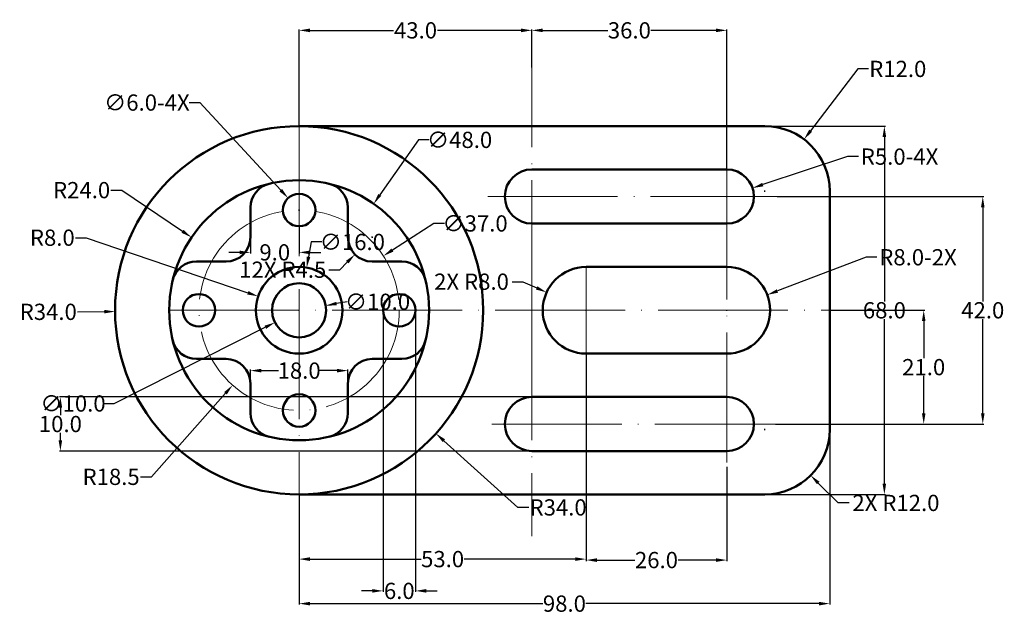
# Model space of a CAD drawing. Units: inches. Extents: x 173 to 355, y 91 to 201.
import ezdxf

# ---------------------------------------------------------------- set-up
doc = ezdxf.new("R2010")
doc.units = ezdxf.units.IN
doc.header["$MEASUREMENT"] = 0
doc.linetypes.add('ACAD_ISO04W100', pattern=[30, 24, -3, 0, -3])
for name, color, linetype, lineweight in [('M-CNTR', 4, 'ACAD_ISO04W100', 18), ('M-DIMS', 2, 'Continuous', 25), ('M-OUTL', 7, 'Continuous', 50)]:
    doc.layers.add(name, color=color, linetype=linetype, lineweight=lineweight)
doc.styles.get("Standard").update_dxf_attribs({"font": 'arial.ttf'})
doc.dimstyles.get("Standard").update_dxf_attribs({"dimtxt": 3, "dimasz": 2, "dimexe": 0.18, "dimexo": 0.0625, "dimgap": 0.09, "dimtad": 0, "dimtih": 1, "dimtoh": 1, "dimdec": 1, "dimzin": 0, "dimdsep": 46, "dimtxsty": 'Standard', "dimcen": 0.09, "dimclrd": 1, "dimclre": 1, "dimadec": 0, "dimazin": 0, "dimtfac": 1, "dimtdec": 1, "dimtofl": 0, "dimtmove": 0, "dimatfit": 3, "dimfxl": 1, "dimtolj": 1, "dimtzin": 0, "dimarcsym": 0})

# ---------------------------------------------------------------- blocks, each defined once
blk = doc.blocks.new('*U1')
blk.add_circle((0, 0), 3)
blk = doc.blocks.new('*U2')
at = {"layer": 'M-OUTL', "color": 0, "linetype": 'ByBlock', "lineweight": -2, "transparency": 16777216}
blk.add_blockref('*U1', (224.3, 165.64), dxfattribs=at)
for p, rotation in [((205.8, 147.14), 90), ((242.8, 147.14), 270), ((224.3, 128.64), 180)]:
    blk.add_blockref('*U1', p, dxfattribs=dict(at, rotation=rotation))
blk = doc.blocks.new('*D3')
at = {"layer": 'Defpoints', "color": 0, "transparency": 16777216}
for p in [(303.3, 198.82), (267.3, 191.92), (303.3, 173.14)]:
    blk.add_point(p, dxfattribs=at)
at = {"layer": 'M-DIMS', "color": 0, "lineweight": -2, "transparency": 16777216}
for p, q in [((267.3, 191.99), (267.3, 199)), ((269.3, 198.82), (281.32, 198.82)), ((301.3, 198.82), (289.28, 198.82)), ((303.3, 173.21), (303.3, 199))]:
    blk.add_line(p, q, dxfattribs=at)
at = {"layer": 'M-DIMS', "color": 0, "transparency": 16777216}
for points in [[(269.3, 199.15), (269.3, 198.48), (267.3, 198.82)], [(301.3, 199.15), (301.3, 198.48), (303.3, 198.82)]]:
    blk.add_solid(points, dxfattribs=at)
at = {"layer": 'M-DIMS', "color": 0, "transparency": 16777216, "insert": (285.3, 198.82), "char_height": 3, "attachment_point": 5}
blk.add_mtext('\\A1;36.0', dxfattribs=at)
blk = doc.blocks.new('*D4')
at = {"layer": 'Defpoints', "color": 0, "transparency": 16777216}
for p in [(267.3, 198.82), (267.3, 191.92), (224.3, 181.14)]:
    blk.add_point(p, dxfattribs=at)
at = {"layer": 'M-DIMS', "color": 0, "lineweight": -2, "transparency": 16777216}
for p, q in [((224.3, 181.21), (224.3, 199)), ((226.3, 198.82), (241.76, 198.82)), ((265.3, 198.82), (249.84, 198.82)), ((267.3, 191.99), (267.3, 199))]:
    blk.add_line(p, q, dxfattribs=at)
at = {"layer": 'M-DIMS', "color": 0, "transparency": 16777216}
for points in [[(226.3, 199.15), (226.3, 198.48), (224.3, 198.82)], [(265.3, 199.15), (265.3, 198.48), (267.3, 198.82)]]:
    blk.add_solid(points, dxfattribs=at)
at = {"layer": 'M-DIMS', "color": 0, "transparency": 16777216, "insert": (245.8, 198.82), "char_height": 3, "attachment_point": 5}
blk.add_mtext('\\A1;43.0', dxfattribs=at)
blk = doc.blocks.new('*D5')
at = {"layer": 'Defpoints', "color": 0, "transparency": 16777216}
for p in [(277.3, 139.14), (224.3, 113.14), (277.3, 101.2)]:
    blk.add_point(p, dxfattribs=at)
at = {"layer": 'M-DIMS', "color": 0, "lineweight": -2, "transparency": 16777216}
for p, q in [((277.3, 139.08), (277.3, 101.02)), ((224.3, 113.08), (224.3, 101.02)), ((226.3, 101.2), (246.82, 101.2)), ((275.3, 101.2), (254.78, 101.2))]:
    blk.add_line(p, q, dxfattribs=at)
at = {"layer": 'M-DIMS', "color": 0, "transparency": 16777216}
for points in [[(226.3, 101.53), (226.3, 100.86), (224.3, 101.2)], [(275.3, 101.53), (275.3, 100.86), (277.3, 101.2)]]:
    blk.add_solid(points, dxfattribs=at)
at = {"layer": 'M-DIMS', "color": 0, "transparency": 16777216, "insert": (250.8, 101.2), "char_height": 3, "attachment_point": 5}
blk.add_mtext('\\A1;53.0', dxfattribs=at)
blk = doc.blocks.new('*D6')
at = {"layer": 'Defpoints', "color": 0, "transparency": 16777216}
for p in [(277.3, 139.14), (303.3, 118.29), (303.3, 101.02)]:
    blk.add_point(p, dxfattribs=at)
at = {"layer": 'M-DIMS', "color": 0, "lineweight": -2, "transparency": 16777216}
for p, q in [((277.3, 139.08), (277.3, 100.84)), ((303.3, 118.22), (303.3, 100.84)), ((279.3, 101.02), (286.29, 101.02)), ((301.3, 101.02), (294.31, 101.02))]:
    blk.add_line(p, q, dxfattribs=at)
at = {"layer": 'M-DIMS', "color": 0, "transparency": 16777216}
for points in [[(279.3, 101.35), (279.3, 100.68), (277.3, 101.02)], [(301.3, 101.35), (301.3, 100.68), (303.3, 101.02)]]:
    blk.add_solid(points, dxfattribs=at)
at = {"layer": 'M-DIMS', "color": 0, "transparency": 16777216, "insert": (290.3, 101.02), "char_height": 3, "attachment_point": 5}
blk.add_mtext('\\A1;26.0', dxfattribs=at)
blk = doc.blocks.new('*D7')
at = {"layer": 'Defpoints', "color": 0, "transparency": 16777216}
for p in [(322.3, 125.14), (224.3, 113.14), (322.3, 92.98)]:
    blk.add_point(p, dxfattribs=at)
at = {"layer": 'M-DIMS', "color": 0, "lineweight": -2, "transparency": 16777216}
for p, q in [((322.3, 125.08), (322.3, 92.8)), ((224.3, 113.08), (224.3, 92.8)), ((226.3, 92.98), (269.32, 92.98)), ((320.3, 92.98), (277.28, 92.98))]:
    blk.add_line(p, q, dxfattribs=at)
at = {"layer": 'M-DIMS', "color": 0, "transparency": 16777216}
for points in [[(226.3, 93.31), (226.3, 92.64), (224.3, 92.98)], [(320.3, 93.31), (320.3, 92.64), (322.3, 92.98)]]:
    blk.add_solid(points, dxfattribs=at)
at = {"layer": 'M-DIMS', "color": 0, "transparency": 16777216, "insert": (273.3, 92.98), "char_height": 3, "attachment_point": 5}
blk.add_mtext('\\A1;98.0', dxfattribs=at)
blk = doc.blocks.new('*D8')
at = {"layer": 'Defpoints', "color": 0, "transparency": 16777216}
for p in [(310.78, 149.99), (303.3, 147.14)]:
    blk.add_point(p, dxfattribs=at)
at = {"layer": 'M-DIMS', "color": 0, "lineweight": -2, "transparency": 16777216}
for p, q in [((329.02, 156.93), (312.65, 150.7)), ((331.02, 156.93), (329.02, 156.93)), ((303.21, 147.14), (303.39, 147.14)), ((303.3, 147.05), (303.3, 147.23))]:
    blk.add_line(p, q, dxfattribs=at)
at = {"layer": 'M-DIMS', "color": 0, "transparency": 16777216}
blk.add_solid([(312.53, 151.01), (312.76, 150.39), (310.78, 149.99)], dxfattribs=at)
at = {"layer": 'M-DIMS', "color": 0, "transparency": 16777216, "insert": (338.62, 156.93), "char_height": 3, "attachment_point": 5}
blk.add_mtext('\\A1;R8.0-2X', dxfattribs=at)
blk = doc.blocks.new('*D9')
at = {"layer": 'Defpoints', "color": 0, "transparency": 16777216}
for p in [(317.57, 178.69), (310.3, 169.14)]:
    blk.add_point(p, dxfattribs=at)
at = {"layer": 'M-DIMS', "color": 0, "lineweight": -2, "transparency": 16777216}
for p, q in [((327.47, 191.7), (318.78, 180.28)), ((329.47, 191.7), (327.47, 191.7)), ((310.3, 169.05), (310.3, 169.23)), ((310.21, 169.14), (310.39, 169.14))]:
    blk.add_line(p, q, dxfattribs=at)
at = {"layer": 'M-DIMS', "color": 0, "transparency": 16777216}
blk.add_solid([(318.51, 180.49), (319.04, 180.08), (317.57, 178.69)], dxfattribs=at)
at = {"layer": 'M-DIMS', "color": 0, "transparency": 16777216, "insert": (334.88, 191.7), "char_height": 3, "attachment_point": 5}
blk.add_mtext('\\A1;R12.0', dxfattribs=at)
blk = doc.blocks.new('*D10')
at = {"layer": 'Defpoints', "color": 0, "transparency": 16777216}
for p in [(308.05, 169.71), (303.3, 168.14)]:
    blk.add_point(p, dxfattribs=at)
at = {"layer": 'M-DIMS', "color": 0, "lineweight": -2, "transparency": 16777216}
for p, q in [((325.61, 175.51), (309.95, 170.34)), ((327.61, 175.51), (325.61, 175.51)), ((303.21, 168.14), (303.39, 168.14)), ((303.3, 168.05), (303.3, 168.23))]:
    blk.add_line(p, q, dxfattribs=at)
at = {"layer": 'M-DIMS', "color": 0, "transparency": 16777216}
blk.add_solid([(309.84, 170.66), (310.05, 170.02), (308.05, 169.71)], dxfattribs=at)
at = {"layer": 'M-DIMS', "color": 0, "transparency": 16777216, "insert": (335.21, 175.51), "char_height": 3, "attachment_point": 5}
blk.add_mtext('\\A1;R5.0-4X', dxfattribs=at)
blk = doc.blocks.new('*D11')
at = {"layer": 'Defpoints', "color": 0, "transparency": 16777216}
for p in [(312.52, 168.14), (312.26, 126.14), (350.58, 126.14)]:
    blk.add_point(p, dxfattribs=at)
at = {"layer": 'M-DIMS', "color": 0, "lineweight": -2, "transparency": 16777216}
for p, q in [((312.58, 168.14), (350.76, 168.14)), ((350.58, 166.14), (350.58, 148.77)), ((350.58, 128.14), (350.58, 145.52)), ((312.32, 126.14), (350.76, 126.14))]:
    blk.add_line(p, q, dxfattribs=at)
at = {"layer": 'M-DIMS', "color": 0, "transparency": 16777216}
for points in [[(350.25, 166.14), (350.91, 166.14), (350.58, 168.14)], [(350.25, 128.14), (350.91, 128.14), (350.58, 126.14)]]:
    blk.add_solid(points, dxfattribs=at)
at = {"layer": 'M-DIMS', "color": 0, "transparency": 16777216, "insert": (350.58, 147.14), "char_height": 3, "attachment_point": 5}
blk.add_mtext('\\A1;42.0', dxfattribs=at)
blk = doc.blocks.new('*D12')
at = {"layer": 'Defpoints', "color": 0, "transparency": 16777216}
for p in [(322.3, 147.14), (312.26, 126.14), (339.67, 126.14)]:
    blk.add_point(p, dxfattribs=at)
at = {"layer": 'M-DIMS', "color": 0, "lineweight": -2, "transparency": 16777216}
for p, q in [((322.36, 147.14), (339.85, 147.14)), ((339.67, 145.14), (339.67, 138.27)), ((339.67, 128.14), (339.67, 135.02)), ((312.32, 126.14), (339.85, 126.14))]:
    blk.add_line(p, q, dxfattribs=at)
at = {"layer": 'M-DIMS', "color": 0, "transparency": 16777216}
for points in [[(339.34, 145.14), (340, 145.14), (339.67, 147.14)], [(339.34, 128.14), (340, 128.14), (339.67, 126.14)]]:
    blk.add_solid(points, dxfattribs=at)
at = {"layer": 'M-DIMS', "color": 0, "transparency": 16777216, "insert": (339.67, 136.64), "char_height": 3, "attachment_point": 5}
blk.add_mtext('\\A1;21.0', dxfattribs=at)
blk = doc.blocks.new('*D13')
at = {"layer": 'Defpoints', "color": 0, "transparency": 16777216}
for p in [(224.3, 162.64), (215.3, 160.64), (224.3, 157.83)]:
    blk.add_point(p, dxfattribs=at)
at = {"layer": 'M-DIMS', "color": 0, "lineweight": -2, "transparency": 16777216}
for p, q in [((224.3, 162.58), (224.3, 157.65)), ((215.3, 160.58), (215.3, 157.65)), ((213.3, 157.83), (211.3, 157.83)), ((226.3, 157.83), (228.3, 157.83))]:
    blk.add_line(p, q, dxfattribs=at)
at = {"layer": 'M-DIMS', "color": 0, "transparency": 16777216}
for points in [[(213.3, 158.16), (213.3, 157.49), (215.3, 157.83)], [(226.3, 158.16), (226.3, 157.49), (224.3, 157.83)]]:
    blk.add_solid(points, dxfattribs=at)
at = {"layer": 'M-DIMS', "color": 0, "transparency": 16777216, "insert": (219.8, 157.83), "char_height": 3, "attachment_point": 5}
blk.add_mtext('\\A1;9.0', dxfattribs=at)
blk = doc.blocks.new('*D14')
at = {"layer": 'Defpoints', "color": 0, "transparency": 16777216}
for p in [(222.26, 167.85), (226.33, 163.44)]:
    blk.add_point(p, dxfattribs=at)
at = {"layer": 'M-DIMS', "color": 0, "lineweight": -2, "transparency": 16777216}
for p, q in [((203.97, 185.49), (205.97, 185.49)), ((205.97, 185.49), (220.91, 169.32)), ((224.21, 165.64), (224.39, 165.64)), ((224.3, 165.55), (224.3, 165.73))]:
    blk.add_line(p, q, dxfattribs=at)
at = {"layer": 'M-DIMS', "color": 0, "transparency": 16777216}
blk.add_solid([(221.15, 169.54), (220.66, 169.09), (222.26, 167.85)], dxfattribs=at)
at = {"layer": 'M-DIMS', "color": 0, "transparency": 16777216, "insert": (196.18, 185.49), "char_height": 3, "attachment_point": 5}
blk.add_mtext('\\A1;∅6.0-4X', dxfattribs=at)
blk = doc.blocks.new('*D15')
at = {"layer": 'Defpoints', "color": 0, "transparency": 16777216}
for p in [(204.42, 160.6), (224.3, 147.14)]:
    blk.add_point(p, dxfattribs=at)
at = {"layer": 'M-DIMS', "color": 0, "lineweight": -2, "transparency": 16777216}
for p, q in [((189.54, 169.32), (191.54, 169.32)), ((191.54, 169.32), (202.77, 161.72)), ((224.21, 147.14), (224.39, 147.14)), ((224.3, 147.05), (224.3, 147.23))]:
    blk.add_line(p, q, dxfattribs=at)
at = {"layer": 'M-DIMS', "color": 0, "transparency": 16777216}
blk.add_solid([(202.95, 161.99), (202.58, 161.44), (204.42, 160.6)], dxfattribs=at)
at = {"layer": 'M-DIMS', "color": 0, "transparency": 16777216, "insert": (184.12, 169.32), "char_height": 3, "attachment_point": 5}
blk.add_mtext('\\A1;R24.0', dxfattribs=at)
blk = doc.blocks.new('*D16')
at = {"layer": 'Defpoints', "color": 0, "transparency": 16777216}
for p in [(190.3, 146.9), (224.3, 147.14)]:
    blk.add_point(p, dxfattribs=at)
at = {"layer": 'M-DIMS', "color": 0, "lineweight": -2, "transparency": 16777216}
for p, q in [((183.37, 146.85), (188.3, 146.89)), ((224.21, 147.14), (224.39, 147.14)), ((224.3, 147.05), (224.3, 147.23))]:
    blk.add_line(p, q, dxfattribs=at)
at = {"layer": 'M-DIMS', "color": 0, "transparency": 16777216}
blk.add_solid([(188.3, 147.22), (188.3, 146.56), (190.3, 146.9)], dxfattribs=at)
at = {"layer": 'M-DIMS', "color": 0, "transparency": 16777216, "insert": (177.96, 146.85), "char_height": 3, "attachment_point": 5}
blk.add_mtext('\\A1;R34.0', dxfattribs=at)
blk = doc.blocks.new('*D17')
at = {"layer": 'Defpoints', "color": 0, "transparency": 16777216}
for p in [(224.3, 147.14), (212.02, 133.31)]:
    blk.add_point(p, dxfattribs=at)
at = {"layer": 'M-DIMS', "color": 0, "lineweight": -2, "transparency": 16777216}
for p, q in [((224.21, 147.14), (224.39, 147.14)), ((224.3, 147.05), (224.3, 147.23)), ((197, 116.39), (210.69, 131.81)), ((195, 116.39), (197, 116.39))]:
    blk.add_line(p, q, dxfattribs=at)
at = {"layer": 'M-DIMS', "color": 0, "transparency": 16777216}
blk.add_solid([(210.44, 132.03), (210.94, 131.59), (212.02, 133.31)], dxfattribs=at)
at = {"layer": 'M-DIMS', "color": 0, "transparency": 16777216, "insert": (189.57, 116.39), "char_height": 3, "attachment_point": 5}
blk.add_mtext('\\A1;R18.5', dxfattribs=at)
blk = doc.blocks.new('*D18')
at = {"layer": 'Defpoints', "color": 0, "transparency": 16777216}
for p in [(216.73, 149.72), (224.3, 147.14)]:
    blk.add_point(p, dxfattribs=at)
at = {"layer": 'M-DIMS', "color": 0, "lineweight": -2, "transparency": 16777216}
for p, q in [((182.96, 160.54), (184.96, 160.54)), ((184.96, 160.54), (214.83, 150.37)), ((224.21, 147.14), (224.39, 147.14)), ((224.3, 147.05), (224.3, 147.23))]:
    blk.add_line(p, q, dxfattribs=at)
at = {"layer": 'M-DIMS', "color": 0, "transparency": 16777216}
blk.add_solid([(214.94, 150.68), (214.72, 150.05), (216.73, 149.72)], dxfattribs=at)
at = {"layer": 'M-DIMS', "color": 0, "transparency": 16777216, "insert": (178.71, 160.54), "char_height": 3, "attachment_point": 5}
blk.add_mtext('\\A1;R8.0', dxfattribs=at)
blk = doc.blocks.new('*D19')
at = {"layer": 'Defpoints', "color": 0, "transparency": 16777216}
for p in [(228.76, 149.39), (219.83, 144.89)]:
    blk.add_point(p, dxfattribs=at)
at = {"layer": 'M-DIMS', "color": 0, "lineweight": -2, "transparency": 16777216}
for p, q in [((224.21, 147.14), (224.39, 147.14)), ((224.3, 147.05), (224.3, 147.23)), ((190.14, 129.93), (218.05, 143.99)), ((188.14, 129.93), (190.14, 129.93))]:
    blk.add_line(p, q, dxfattribs=at)
at = {"layer": 'M-DIMS', "color": 0, "transparency": 16777216}
blk.add_solid([(217.9, 144.29), (218.2, 143.7), (219.83, 144.89)], dxfattribs=at)
at = {"layer": 'M-DIMS', "color": 0, "transparency": 16777216, "insert": (182.53, 129.93), "char_height": 3, "attachment_point": 5}
blk.add_mtext('\\A1;∅10.0', dxfattribs=at)
blk = doc.blocks.new('*D20')
at = {"layer": 'Defpoints', "color": 0, "transparency": 16777216}
for p in [(233.3, 136), (215.3, 133.64), (233.3, 133.64)]:
    blk.add_point(p, dxfattribs=at)
at = {"layer": 'M-DIMS', "color": 0, "lineweight": -2, "transparency": 16777216}
for p, q in [((215.3, 133.71), (215.3, 136.18)), ((217.3, 136), (220.46, 136)), ((231.3, 136), (228.14, 136)), ((233.3, 133.71), (233.3, 136.18))]:
    blk.add_line(p, q, dxfattribs=at)
at = {"layer": 'M-DIMS', "color": 0, "transparency": 16777216}
for points in [[(217.3, 136.33), (217.3, 135.66), (215.3, 136)], [(231.3, 136.33), (231.3, 135.66), (233.3, 136)]]:
    blk.add_solid(points, dxfattribs=at)
at = {"layer": 'M-DIMS', "color": 0, "transparency": 16777216, "insert": (224.3, 136), "char_height": 3, "attachment_point": 5}
blk.add_mtext('\\A1;18.0', dxfattribs=at)
blk = doc.blocks.new('HUB-INTERLOBE-RELIEF')
for p, q in [((3.46, 7.96), (3.46, 13.44)), ((7.96, 3.46), (13.44, 3.46))]:
    blk.add_line(p, q)
for centre, start, end in [((-1.04, 13.44), 0, 76.6576), ((7.96, 7.96), 180, 270), ((13.44, -1.04), 13.3424, 90)]:
    blk.add_arc(centre, 4.5, start, end)
blk = doc.blocks.new('GUIDE-SLOT-NARROW')
blk.add_lwpolyline([(41, 10), (5, 10, 1), (5, 0), (41, 0, 1)], format="xyb", close=True)
blk = doc.blocks.new('*D23')
at = {"layer": 'Defpoints', "color": 0, "transparency": 16777216}
for p in [(310.3, 181.14), (310.3, 113.14), (332.4, 113.14)]:
    blk.add_point(p, dxfattribs=at)
at = {"layer": 'M-DIMS', "color": 1, "lineweight": -2, "transparency": 16777216}
for p, q in [((310.36, 181.14), (332.58, 181.14)), ((332.4, 179.14), (332.4, 148.77)), ((332.4, 115.14), (332.4, 145.52)), ((310.36, 113.14), (332.58, 113.14))]:
    blk.add_line(p, q, dxfattribs=at)
at = {"layer": 'M-DIMS', "color": 1, "transparency": 16777216}
for points in [[(332.07, 179.14), (332.73, 179.14), (332.4, 181.14)], [(332.07, 115.14), (332.73, 115.14), (332.4, 113.14)]]:
    blk.add_solid(points, dxfattribs=at)
at = {"layer": 'M-DIMS', "color": 0, "transparency": 16777216, "insert": (332.4, 147.14), "char_height": 3, "attachment_point": 5}
blk.add_mtext('\\A1;68.0', dxfattribs=at)
blk = doc.blocks.new('*D24')
at = {"layer": 'Defpoints', "color": 0, "transparency": 16777216}
for p in [(239.8, 147.14), (245.8, 147.14), (245.8, 95.33)]:
    blk.add_point(p, dxfattribs=at)
at = {"layer": 'M-DIMS', "color": 1, "lineweight": -2, "transparency": 16777216}
for p, q in [((239.8, 147.08), (239.8, 95.15)), ((245.8, 147.08), (245.8, 95.15)), ((237.8, 95.33), (235.8, 95.33)), ((247.8, 95.33), (249.8, 95.33))]:
    blk.add_line(p, q, dxfattribs=at)
at = {"layer": 'M-DIMS', "color": 1, "transparency": 16777216}
for points in [[(237.8, 95.67), (237.8, 95), (239.8, 95.33)], [(247.8, 95.67), (247.8, 95), (245.8, 95.33)]]:
    blk.add_solid(points, dxfattribs=at)
at = {"layer": 'M-DIMS', "color": 0, "transparency": 16777216, "insert": (242.8, 95.33), "char_height": 3, "attachment_point": 5}
blk.add_mtext('\\A1;6.0', dxfattribs=at)
blk = doc.blocks.new('*D25')
at = {"layer": 'Defpoints', "color": 0, "transparency": 16777216}
for p in [(180.2, 131.14), (267.3, 131.14), (267.3, 121.14)]:
    blk.add_point(p, dxfattribs=at)
at = {"layer": 'M-DIMS', "color": 1, "lineweight": -2, "transparency": 16777216}
for p, q in [((267.24, 131.14), (180.02, 131.14)), ((180.2, 129.14), (180.2, 127.77)), ((180.2, 123.14), (180.2, 124.52)), ((267.24, 121.14), (180.02, 121.14))]:
    blk.add_line(p, q, dxfattribs=at)
at = {"layer": 'M-DIMS', "color": 1, "transparency": 16777216}
for points in [[(179.87, 129.14), (180.53, 129.14), (180.2, 131.14)], [(179.87, 123.14), (180.53, 123.14), (180.2, 121.14)]]:
    blk.add_solid(points, dxfattribs=at)
at = {"layer": 'M-DIMS', "color": 0, "transparency": 16777216, "insert": (180.2, 126.14), "char_height": 3, "attachment_point": 5}
blk.add_mtext('\\A1;10.0', dxfattribs=at)
blk = doc.blocks.new('*D26')
at = {"layer": 'Defpoints', "color": 0, "transparency": 16777216}
for p in [(224.3, 147.14), (249.56, 124.39)]:
    blk.add_point(p, dxfattribs=at)
at = {"layer": 'M-DIMS', "color": 1, "lineweight": -2, "transparency": 16777216}
for p, q in [((224.21, 147.14), (224.39, 147.14)), ((224.3, 147.05), (224.3, 147.23)), ((264.72, 110.74), (251.05, 123.05)), ((266.72, 110.74), (264.72, 110.74))]:
    blk.add_line(p, q, dxfattribs=at)
at = {"layer": 'M-DIMS', "color": 1, "transparency": 16777216}
blk.add_solid([(251.27, 123.3), (250.83, 122.8), (249.56, 124.39)], dxfattribs=at)
at = {"layer": 'M-DIMS', "color": 0, "transparency": 16777216, "insert": (272.14, 110.74), "char_height": 3, "attachment_point": 5}
blk.add_mtext('\\A1;R34.0', dxfattribs=at)
blk = doc.blocks.new('*D27')
at = {"layer": 'Defpoints', "color": 0, "transparency": 16777216}
for p in [(238.06, 166.8), (210.53, 127.48)]:
    blk.add_point(p, dxfattribs=at)
at = {"layer": 'M-DIMS', "color": 1, "lineweight": -2, "transparency": 16777216}
for p, q in [((246.32, 178.6), (239.21, 168.44)), ((248.32, 178.6), (246.32, 178.6)), ((224.21, 147.14), (224.39, 147.14)), ((224.3, 147.05), (224.3, 147.23))]:
    blk.add_line(p, q, dxfattribs=at)
at = {"layer": 'M-DIMS', "color": 1, "transparency": 16777216}
blk.add_solid([(238.94, 168.63), (239.48, 168.25), (238.06, 166.8)], dxfattribs=at)
at = {"layer": 'M-DIMS', "color": 0, "transparency": 16777216, "insert": (253.94, 178.6), "char_height": 3, "attachment_point": 5}
blk.add_mtext('\\A1;∅48.0', dxfattribs=at)
blk = doc.blocks.new('*D28')
at = {"layer": 'Defpoints', "color": 0, "transparency": 16777216}
for p in [(239.85, 157.16), (208.75, 137.13)]:
    blk.add_point(p, dxfattribs=at)
at = {"layer": 'M-DIMS', "color": 1, "lineweight": -2, "transparency": 16777216}
for p, q in [((249.18, 163.17), (241.53, 158.25)), ((251.18, 163.17), (249.18, 163.17)), ((224.21, 147.14), (224.39, 147.14)), ((224.3, 147.05), (224.3, 147.23))]:
    blk.add_line(p, q, dxfattribs=at)
at = {"layer": 'M-DIMS', "color": 1, "transparency": 16777216}
blk.add_solid([(241.35, 158.53), (241.71, 157.97), (239.85, 157.16)], dxfattribs=at)
at = {"layer": 'M-DIMS', "color": 0, "transparency": 16777216, "insert": (256.8, 163.17), "char_height": 3, "attachment_point": 5}
blk.add_mtext('\\A1;∅37.0', dxfattribs=at)
blk = doc.blocks.new('*D29')
at = {"layer": 'Defpoints', "color": 0, "transparency": 16777216}
for p in [(225.69, 155.02), (222.91, 139.27)]:
    blk.add_point(p, dxfattribs=at)
at = {"layer": 'M-DIMS', "color": 1, "lineweight": -2, "transparency": 16777216}
for p, q in [((226.52, 159.75), (226.04, 156.99)), ((228.52, 159.75), (226.52, 159.75)), ((224.21, 147.14), (224.39, 147.14)), ((224.3, 147.05), (224.3, 147.23))]:
    blk.add_line(p, q, dxfattribs=at)
at = {"layer": 'M-DIMS', "color": 1, "transparency": 16777216}
blk.add_solid([(225.71, 157.05), (226.36, 156.93), (225.69, 155.02)], dxfattribs=at)
at = {"layer": 'M-DIMS', "color": 0, "transparency": 16777216, "insert": (234.13, 159.75), "char_height": 3, "attachment_point": 5}
blk.add_mtext('\\A1;∅16.0', dxfattribs=at)
blk = doc.blocks.new('*D30')
at = {"layer": 'Defpoints', "color": 0, "transparency": 16777216}
for p in [(229.22, 148.01), (219.37, 146.28)]:
    blk.add_point(p, dxfattribs=at)
at = {"layer": 'M-DIMS', "color": 1, "lineweight": -2, "transparency": 16777216}
for p, q in [((233.16, 148.71), (231.19, 148.36)), ((224.21, 147.14), (224.39, 147.14)), ((224.3, 147.05), (224.3, 147.23))]:
    blk.add_line(p, q, dxfattribs=at)
at = {"layer": 'M-DIMS', "color": 1, "transparency": 16777216}
blk.add_solid([(231.13, 148.69), (231.25, 148.03), (229.22, 148.01)], dxfattribs=at)
at = {"layer": 'M-DIMS', "color": 0, "transparency": 16777216, "insert": (238.78, 148.71), "char_height": 3, "attachment_point": 5}
blk.add_mtext('\\A1;∅10.0', dxfattribs=at)
blk = doc.blocks.new('*D31')
at = {"layer": 'Defpoints', "color": 0, "transparency": 16777216}
for p in [(237.8, 160.64), (234.62, 157.46)]:
    blk.add_point(p, dxfattribs=at)
at = {"layer": 'M-DIMS', "color": 1, "lineweight": -2, "transparency": 16777216}
for p, q in [((237.71, 160.64), (237.89, 160.64)), ((237.8, 160.55), (237.8, 160.73)), ((229.79, 154.63), (231.79, 154.63)), ((231.79, 154.63), (233.2, 156.05))]:
    blk.add_line(p, q, dxfattribs=at)
at = {"layer": 'M-DIMS', "color": 1, "transparency": 16777216}
blk.add_solid([(232.97, 156.28), (233.44, 155.81), (234.62, 157.46)], dxfattribs=at)
at = {"layer": 'M-DIMS', "color": 0, "transparency": 16777216, "insert": (221.27, 154.63), "char_height": 3, "attachment_point": 5}
blk.add_mtext('\\A1;12X R4.5', dxfattribs=at)
blk = doc.blocks.new('*D32')
at = {"layer": 'Defpoints', "color": 0, "transparency": 16777216}
for p in [(310.3, 125.14), (318.78, 116.66)]:
    blk.add_point(p, dxfattribs=at)
at = {"layer": 'M-DIMS', "color": 1, "lineweight": -2, "transparency": 16777216}
for p, q in [((310.21, 125.14), (310.39, 125.14)), ((310.3, 125.05), (310.3, 125.23)), ((323.88, 111.57), (320.2, 115.24)), ((325.88, 111.57), (323.88, 111.57))]:
    blk.add_line(p, q, dxfattribs=at)
at = {"layer": 'M-DIMS', "color": 1, "transparency": 16777216}
blk.add_solid([(320.43, 115.48), (319.96, 115.01), (318.78, 116.66)], dxfattribs=at)
at = {"layer": 'M-DIMS', "color": 0, "transparency": 16777216, "insert": (334.54, 111.57), "char_height": 3, "attachment_point": 5}
blk.add_mtext('\\A1;2X R12.0', dxfattribs=at)
blk = doc.blocks.new('*D33')
at = {"layer": 'Defpoints', "color": 0, "transparency": 16777216}
for p in [(270.01, 150.44), (277.3, 147.14)]:
    blk.add_point(p, dxfattribs=at)
at = {"layer": 'M-DIMS', "color": 1, "lineweight": -2, "transparency": 16777216}
for p, q in [((263.64, 152.42), (265.64, 152.42)), ((265.64, 152.42), (268.19, 151.27)), ((277.21, 147.14), (277.39, 147.14)), ((277.3, 147.05), (277.3, 147.23))]:
    blk.add_line(p, q, dxfattribs=at)
at = {"layer": 'M-DIMS', "color": 1, "transparency": 16777216}
blk.add_solid([(268.33, 151.57), (268.05, 150.97), (270.01, 150.44)], dxfattribs=at)
at = {"layer": 'M-DIMS', "color": 0, "transparency": 16777216, "insert": (256.14, 152.42), "char_height": 3, "attachment_point": 5}
blk.add_mtext('\\A1;2X R8.0', dxfattribs=at)

msp = doc.modelspace()

# ---------------------------------------------------------------- linework, layer by layer
at = {"layer": 'M-CNTR'}
for p, q in [((267.3, 147.14), (267.3, 191.92)), ((224.3, 181.14), (224.3, 113.14)), ((303.3, 173.14), (303.3, 118.29)), ((259.13, 168.14), (312.52, 168.14)), ((277.3, 155.14), (277.3, 139.14)), ((200.3, 147.14), (322.3, 147.14)), ((267.3, 147.14), (267.3, 105.43)), ((259.88, 126.14), (312.26, 126.14))]:
    msp.add_line(p, q, dxfattribs=at)
msp.add_circle((224.3, 147.14), 18.5, dxfattribs=at)
at = {"layer": 'M-OUTL'}
for p, q in [((224.3, 181.14), (310.3, 181.14)), ((322.3, 125.14), (322.3, 169.14)), ((277.3, 155.14), (303.3, 155.14)), ((277.3, 139.14), (303.3, 139.14)), ((224.3, 113.14), (310.3, 113.14))]:
    msp.add_line(p, q, dxfattribs=at)
for radius in [34, 24, 8, 5]:
    msp.add_circle((224.3, 147.14), radius, dxfattribs=at)
for centre, radius, start, end in [((310.3, 169.14), 12, 0, 90), ((277.3, 147.14), 8, 90, 270), ((303.3, 147.14), 8, 270, 90), ((310.3, 125.14), 12, 270, 0)]:
    msp.add_arc(centre, radius, start, end, dxfattribs=at)

# ---------------------------------------------------------------- block references
for name, p in [('GUIDE-SLOT-NARROW', (262.3, 163.14)), ('HUB-INTERLOBE-RELIEF', (229.84, 152.68)), ('*U2', (0, 0))]:
    msp.add_blockref(name, p, dxfattribs=at)
for p, rotation in [((218.76, 152.68), 89.99999999999974), ((218.76, 141.61), 180), ((229.84, 141.61), 269.9999999999998)]:
    msp.add_blockref('HUB-INTERLOBE-RELIEF', p, dxfattribs=dict(at, rotation=rotation))
at = {"layer": 'M-OUTL', "extrusion": (0, 0, -1), "zscale": -1, "rotation": 180}
msp.add_blockref('GUIDE-SLOT-NARROW', (-262.3, 131.14), dxfattribs=at)

# ---------------------------------------------------------------- dimensions: what is measured, and where the dimension line sits
at = {"layer": 'M-DIMS'}
for base, p1, p2, override, picture, middle in [((267.3, 198.82), (224.3, 181.14), (267.3, 191.92), {"dimclrd": 0, "dimclre": 0, "dimclrt": 0}, '*D4', (245.8, 198.82)), ((303.3, 198.82), (267.3, 191.92), (303.3, 173.14), {"dimclrd": 0, "dimclre": 0, "dimclrt": 0}, '*D3', (285.3, 198.82)), ((224.3, 157.83), (215.3, 160.64), (224.3, 162.64), {"dimclrd": 0, "dimclre": 0, "dimclrt": 0}, '*D13', (219.8, 157.83)), ((245.8, 95.33), (239.8, 147.14), (245.8, 147.14), {"dimdec": 1, "dimlfac": 1, "dimrnd": 0, "dimzin": 0, "dimdsep": 46, "dimlunit": 2}, '*D24', (242.8, 95.33)), ((277.3, 101.2), (224.3, 113.14), (277.3, 139.14), {"dimclrd": 0, "dimclre": 0, "dimclrt": 0}, '*D5', (250.8, 101.2)), ((303.3, 101.02), (277.3, 139.14), (303.3, 118.29), {"dimclrd": 0, "dimclre": 0, "dimclrt": 0}, '*D6', (290.3, 101.02)), ((233.3, 136), (215.3, 133.64), (233.3, 133.64), {"dimclrd": 0, "dimclre": 0, "dimclrt": 0}, '*D20', (224.3, 136)), ((322.3, 92.98), (224.3, 113.14), (322.3, 125.14), {"dimclrd": 0, "dimclre": 0, "dimclrt": 0}, '*D7', (273.3, 92.98))]:
    dim = msp.add_linear_dim(base=base, p1=p1, p2=p2, dimstyle='Standard', override=override, dxfattribs=at)
    dim.commit()
    dim.dimension.update_dxf_attribs({"geometry": picture, "text_midpoint": middle})
for center, mpoint, override, picture, middle in [((310.3, 169.14), (317.57, 178.69), {"dimclrd": 0, "dimclre": 0, "dimclrt": 0}, '*D9', (334.88, 191.7)), ((224.3, 147.14), (204.42, 160.6), {"dimclrd": 0, "dimclre": 0, "dimclrt": 0}, '*D15', (184.12, 169.32)), ((224.3, 147.14), (216.73, 149.72), {"dimclrd": 0, "dimclre": 0, "dimclrt": 0}, '*D18', (178.71, 160.54)), ((224.3, 147.14), (190.3, 146.9), {"dimclrd": 0, "dimclre": 0, "dimclrt": 0}, '*D16', (183.37, 146.85)), ((224.3, 147.14), (212.02, 133.31), {"dimclrd": 0, "dimclre": 0, "dimclrt": 0}, '*D17', (189.57, 116.39)), ((224.3, 147.14), (249.56, 124.39), {"dimdec": 1, "dimlfac": 1, "dimrnd": 0, "dimzin": 0, "dimdsep": 46, "dimlunit": 2}, '*D26', (272.14, 110.74))]:
    dim = msp.add_radius_dim(center=center, mpoint=mpoint, dimstyle='Standard', override=override, dxfattribs=at)
    dim.commit()
    dim.dimension.update_dxf_attribs({"geometry": picture, "text_midpoint": middle, "dimtype": 164})
dim = msp.add_diameter_dim_2p(p1=(226.33, 163.44), p2=(222.26, 167.85), text='<>-4X', dimstyle='Standard', override={"dimclrd": 0, "dimclre": 0, "dimclrt": 0}, dxfattribs=at)
dim.commit()
dim.dimension.update_dxf_attribs({"geometry": '*D14', "text_midpoint": (196.18, 185.49), "dimtype": 163})
for p1, p2, override, picture, middle in [((210.53, 127.48), (238.06, 166.8), {"dimdec": 1, "dimlfac": 1, "dimrnd": 0, "dimzin": 0, "dimdsep": 46, "dimlunit": 2}, '*D27', (253.94, 178.6)), ((208.75, 137.13), (239.85, 157.16), {"dimdec": 1, "dimlfac": 1, "dimrnd": 0, "dimzin": 0, "dimdsep": 46, "dimlunit": 2}, '*D28', (256.8, 163.17)), ((222.91, 139.27), (225.69, 155.02), {"dimdec": 1, "dimlfac": 1, "dimrnd": 0, "dimzin": 0, "dimdsep": 46, "dimlunit": 2}, '*D29', (234.13, 159.75)), ((228.76, 149.39), (219.83, 144.89), {"dimclrd": 0, "dimclre": 0, "dimclrt": 0}, '*D19', (182.53, 129.93)), ((219.37, 146.28), (229.22, 148.01), {"dimdec": 1, "dimlfac": 1, "dimrnd": 0, "dimzin": 0, "dimdsep": 46, "dimlunit": 2}, '*D30', (233.16, 148.71))]:
    dim = msp.add_diameter_dim_2p(p1=p1, p2=p2, dimstyle='Standard', override=override, dxfattribs=at)
    dim.commit()
    dim.dimension.update_dxf_attribs({"geometry": picture, "text_midpoint": middle, "dimtype": 163})
for base, p1, p2, override, picture, middle in [((332.4, 113.14), (310.3, 181.14), (310.3, 113.14), {"dimdec": 1, "dimlfac": 1, "dimrnd": 0, "dimzin": 0, "dimdsep": 46, "dimlunit": 2}, '*D23', (332.4, 147.14)), ((350.58, 126.14), (312.52, 168.14), (312.26, 126.14), {"dimclrd": 0, "dimclre": 0, "dimclrt": 0}, '*D11', (350.58, 147.14)), ((339.67, 126.14), (322.3, 147.14), (312.26, 126.14), {"dimclrd": 0, "dimclre": 0, "dimclrt": 0}, '*D12', (339.67, 136.64)), ((180.2, 131.14), (267.3, 121.14), (267.3, 131.14), {"dimdec": 1, "dimlfac": 1, "dimrnd": 0, "dimzin": 0, "dimdsep": 46, "dimlunit": 2}, '*D25', (180.2, 126.14))]:
    dim = msp.add_linear_dim(base=base, p1=p1, p2=p2, angle=90, dimstyle='Standard', override=override, dxfattribs=at)
    dim.commit()
    dim.dimension.update_dxf_attribs({"geometry": picture, "text_midpoint": middle})
for center, mpoint, text, override, picture, middle in [((303.3, 168.14), (308.05, 169.71), '<>-4X', {"dimclrd": 0, "dimclre": 0, "dimclrt": 0}, '*D10', (335.21, 175.51)), ((303.3, 147.14), (310.78, 149.99), '<>-2X', {"dimclrd": 0, "dimclre": 0, "dimclrt": 0}, '*D8', (338.62, 156.93)), ((277.3, 147.14), (270.01, 150.44), '2X <>', {"dimdec": 1, "dimlfac": 1, "dimrnd": 0, "dimzin": 0, "dimdsep": 46, "dimlunit": 2}, '*D33', (256.14, 152.42)), ((310.3, 125.14), (318.78, 116.66), '2X <>', {"dimdec": 1, "dimlfac": 1, "dimrnd": 0, "dimzin": 0, "dimdsep": 46, "dimlunit": 2}, '*D32', (334.54, 111.57))]:
    dim = msp.add_radius_dim(center=center, mpoint=mpoint, text=text, dimstyle='Standard', override=override, dxfattribs=at)
    dim.commit()
    dim.dimension.update_dxf_attribs({"geometry": picture, "text_midpoint": middle, "dimtype": 164})
dim = msp.add_radius_dim(center=(237.8, 160.64), mpoint=(234.62, 157.46), text='12X <>', dimstyle='Standard', override={"dimdec": 1, "dimlfac": 1, "dimrnd": 0, "dimzin": 0, "dimdsep": 46, "dimlunit": 2}, dxfattribs=at)
dim.commit()
dim.dimension.update_dxf_attribs({"geometry": '*D31', "text_midpoint": (221.27, 154.63)})

doc.saveas('drawing.dxf')
